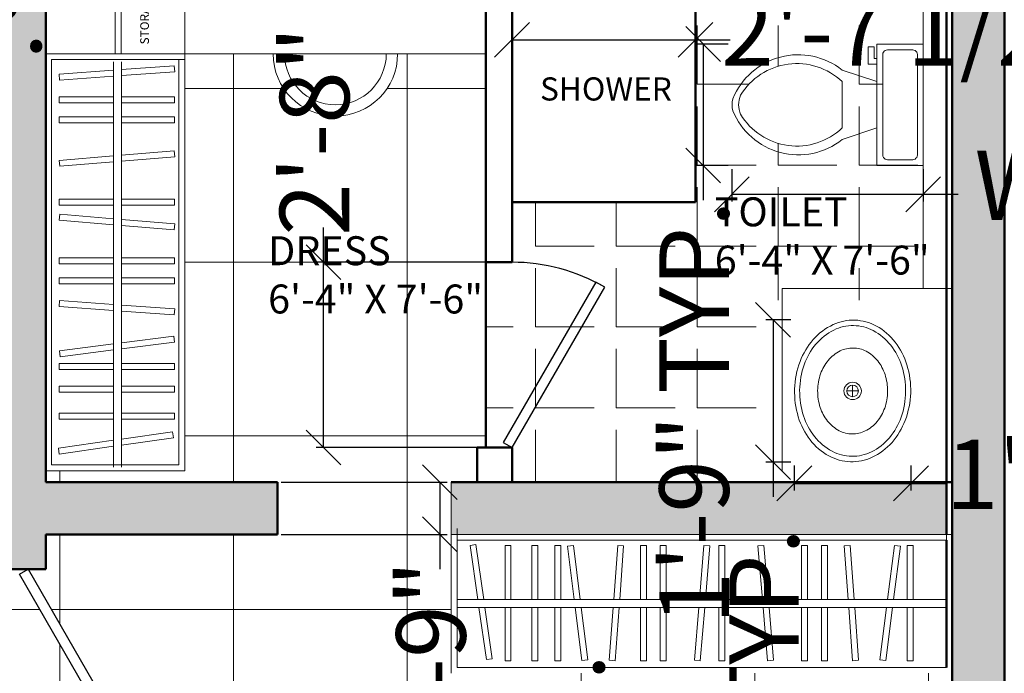
# Model space of a CAD drawing. Units: inches. Extents: x 2371 to 3019, y 129 to 700.
# Tile 12 of 14: x 2753 to 2923, y 499 to 612. Entities that reach past the tile are written whole.
import ezdxf

# ---------------------------------------------------------------- set-up
doc = ezdxf.new("R2010")
doc.units = ezdxf.units.IN
for name, color, linetype, lineweight in [('A-ANNO-DIMS', 2, 'Continuous', 18), ('A-AREA-IDEN', 7, 'Continuous', 25), ('A-DOOR', 4, 'Continuous', 25), ('A-FLOR-FIXT', 8, 'Continuous', 18), ('A-FLOR-PATT', 252, 'Continuous', 13), ('A-FURN', 8, 'Continuous', 18), ('A-WALL', 7, 'Continuous', 50), ('A-WALL-PATT', 8, 'Continuous', 13)]:
    doc.layers.add(name, color=color, linetype=linetype, lineweight=lineweight)
doc.styles.get("Standard").update_dxf_attribs({"font": 'arial.ttf'})
doc.dimstyles.new('ISO-25', dxfattribs={"dimtxt": 12, "dimasz": 6, "dimexe": 1.25, "dimexo": 0.625, "dimtad": 0, "dimdec": 1, "dimlunit": 3, "dimtxsty": 'Standard', "dimblk": 'OBLIQUE', "dimblk1": 'ORIGIN2', "dimblk2": 'OBLIQUE', "dimcen": 2.5, "dimadec": 0, "dimazin": 0, "dimtfac": 1, "dimtdec": 1, "dimtmove": 0, "dimatfit": 3, "dimldrblk": 'OBLIQUE', "dimfxl": 1, "dimarcsym": 0})

# ---------------------------------------------------------------- blocks, each defined once
blk = doc.blocks.new('*U3')
for p, q in [((0, 0), (0, -6)), ((-32, 0), (-32, -6))]:
    blk.add_line(p, q)
blk.add_lwpolyline([(0, 0), (-27.71, 16), (-28.59, 14.48), (-0.88, -1.52)], close=True)
blk.add_arc((0, 0), 32, 150, 180)
blk = doc.blocks.new('*U10')
for p, q in [((0, 0), (0, -6)), ((36, 0), (36, -6))]:
    blk.add_line(p, q)
blk.add_lwpolyline([(0, 0), (31.18, 18), (32.05, 16.48), (0.87, -1.52)], close=True)
blk.add_arc((0, 0), 36, 0, 30)
blk = doc.blocks.new('Sink - Oval top')
for p, q in [((-1, 0), (1, 0)), ((0, 1), (0, -1))]:
    blk.add_line(p, q)
for points in [[(-12.23, 0.39, 0.117634), (-11.46, -3.36, 0.104469), (-8.88, -6.8, 0.090016), (-5.08, -9.07, 0.08192), (-0.32, -10.02, 0.08192), (4.49, -9.38, 0.090016), (8.42, -7.36, 0.104469), (11.22, -4.09, 0.117634), (12.23, -0.39, 0.117634), (11.46, 3.36, 0.104469), (8.88, 6.8, 0.090016), (5.08, 9.07, 0.08192), (0.32, 10.02, 0.08192), (-4.49, 9.38, 0.090016), (-8.42, 7.36, 0.104469), (-11.22, 4.09, 0.117634)], [(-11.29, 0.16, 0.118622), (-10.52, -3.25, 0.104678), (-8.07, -6.36, 0.089562), (-4.54, -8.37, 0.081185), (-0.13, -9.15, 0.081185), (4.3, -8.49, 0.089562), (7.89, -6.58, 0.104678), (10.42, -3.55, 0.118622), (11.29, -0.16, 0.118622), (10.52, 3.25, 0.104678), (8.07, 6.36, 0.089562), (4.54, 8.37, 0.081185), (0.13, 9.15, 0.081185), (-4.3, 8.49, 0.089562), (-7.89, 6.58, 0.104678), (-10.42, 3.55, 0.118622)], [(-7.42, 0.08, 0.118283), (-6.91, -2.17, 0.104607), (-5.29, -4.21, 0.089718), (-2.97, -5.53, 0.081436), (-0.07, -6.04, 0.081436), (2.84, -5.59, 0.089718), (5.2, -4.33, 0.104607), (6.86, -2.32, 0.118283), (7.42, -0.08, 0.118283), (6.91, 2.17, 0.104607), (5.29, 4.21, 0.089718), (2.97, 5.53, 0.081436), (0.07, 6.04, 0.081436), (-2.84, 5.59, 0.089718), (-5.2, 4.33, 0.104607), (-6.86, 2.32, 0.118283)]]:
    blk.add_lwpolyline(points, format="xyb", close=True)
for radius in [1.5, 1]:
    blk.add_circle((0, 0), radius)
blk = doc.blocks.new('Toilet - top')
for p, q in [((9.5, -6), (9.5, -2)), ((-8, -8.5), (-8, -8)), ((-7, -8), (-7, -9.5)), ((-4, -8), (-6, -14)), ((4, -8), (6, -14)), ((-10, -8.5), (-8, -8.5)), ((-10, -9.5), (-10, -8.5)), ((-7, -9.5), (-10, -9.5)), ((4, -14), (-4, -14))]:
    blk.add_line(p, q)
blk.add_lwpolyline([(10.5, -8), (10.5, 0), (-10.5, 0), (-10.5, -8)], close=True)
for points in [[(8.5, -1), (-8.5, -1)], [(-9.5, -2), (-9.5, -6)], [(-8.5, -7), (8.5, -7)]]:
    blk.add_lwpolyline(points)
for centre, radius, start, end in [((-8.62, -1.88), 0.884, 81.8699, 188.1301), ((8.62, -1.88), 0.884, 351.8699, 98.1301), ((-8.62, -6.12), 0.884, 171.8699, 278.1301), ((8.62, -6.12), 0.884, 261.8699, 8.1301), ((3.52, -21.58), 12.17, 141.4691, 247.9714), ((4.2, -21.82), 11.33, 136.3677, 238.9468), ((-3.52, -21.58), 12.17, 292.0284, 38.5307), ((-4.2, -21.82), 11.33, 301.053, 43.6321), ((0, -27.88), 4, 245.7318, 294.2682), ((0, -29), 4, 254.8605, 285.1395)]:
    blk.add_arc(centre, radius, start, end)
blk = doc.blocks.new('_Oblique')
at = {"color": 0, "linetype": 'ByBlock', "lineweight": -2}
blk.add_line((-0.5, -0.5), (0.5, 0.5), dxfattribs=at)
blk = doc.blocks.new('*D25')
at = {"layer": 'A-ANNO-DIMS', "color": 0, "lineweight": -2, "transparency": 16777216}
for p, q in [((2849.61, 422.48), (2849.61, 428.48)), ((2838.23, 422.48), (2850.86, 422.48)), ((2849.61, 362.48), (2849.61, 422.48)), ((2838.23, 362.48), (2850.86, 362.48))]:
    blk.add_line(p, q, dxfattribs=at)
at = {"layer": 'Defpoints', "color": 0, "lineweight": 25, "transparency": 16777216}
for p in [(2837.61, 422.48), (2849.61, 422.48), (2837.61, 362.48)]:
    blk.add_point(p, dxfattribs=at)
at = {"layer": 'A-ANNO-DIMS', "color": 0, "lineweight": -2, "transparency": 16777216, "xscale": 6, "yscale": 6, "zscale": 6}
for p, rotation in [((2849.61, 422.48), 90), ((2849.61, 362.48), 270)]:
    blk.add_blockref('_Oblique', p, dxfattribs=dict(at, rotation=rotation))
at = {"layer": 'A-ANNO-DIMS', "color": 0, "transparency": 16777216, "insert": (2849.61, 465.67), "char_height": 12, "attachment_point": 5, "rotation": 90}
blk.add_mtext('5\'-0" TYP.', dxfattribs=at)
blk = doc.blocks.new('_Origin2')
at = {"color": 0, "linetype": 'ByBlock', "lineweight": -2}
blk.add_line((-0.5, 0), (-1, 0), dxfattribs=at)
for radius in [0.5, 0.25]:
    blk.add_circle((0, 0), radius, dxfattribs=at)
blk = doc.blocks.new('*D26')
at = {"layer": 'A-ANNO-DIMS', "color": 0, "lineweight": -2, "transparency": 16777216}
for p, q in [((2886.23, 560.02), (2881.92, 560.02)), ((2883.17, 560.02), (2883.17, 535.47)), ((2886.23, 535.47), (2881.92, 535.47)), ((2883.17, 535.47), (2883.17, 529.47))]:
    blk.add_line(p, q, dxfattribs=at)
at = {"layer": 'Defpoints', "color": 0, "lineweight": 25, "transparency": 16777216}
for p in [(2886.85, 560.02), (2883.17, 535.47), (2886.85, 535.47)]:
    blk.add_point(p, dxfattribs=at)
at = {"layer": 'A-ANNO-DIMS', "color": 0, "lineweight": -2, "transparency": 16777216, "xscale": 6, "yscale": 6, "zscale": 6}
for p, rotation in [((2883.17, 560.02), 90), ((2883.17, 535.47), 270)]:
    blk.add_blockref('_Oblique', p, dxfattribs=dict(at, rotation=rotation))
at = {"layer": 'A-ANNO-DIMS', "color": 0, "transparency": 16777216, "insert": (2883.17, 423.09), "char_height": 12, "attachment_point": 5, "rotation": 90}
blk.add_mtext('WASH BASIN 2\'-0 1/2" TYP.', dxfattribs=at)
blk = doc.blocks.new('*D27')
at = {"layer": 'A-ANNO-DIMS', "color": 0, "lineweight": -2, "transparency": 16777216}
for p, q in [((2886.85, 534.85), (2886.85, 530.54)), ((2906.99, 534.85), (2906.99, 530.54)), ((2886.85, 531.79), (2906.99, 531.79)), ((2906.99, 531.79), (2912.99, 531.79))]:
    blk.add_line(p, q, dxfattribs=at)
at = {"layer": 'Defpoints', "color": 0, "lineweight": 25, "transparency": 16777216}
for p in [(2886.85, 535.47), (2906.99, 535.47), (2906.99, 531.79)]:
    blk.add_point(p, dxfattribs=at)
at = {"layer": 'A-ANNO-DIMS', "color": 0, "lineweight": -2, "transparency": 16777216, "xscale": 6, "yscale": 6, "zscale": 6, "rotation": 180}
blk.add_blockref('_Oblique', (2886.85, 531.79), dxfattribs=at)
at = {"layer": 'A-ANNO-DIMS', "color": 0, "lineweight": -2, "transparency": 16777216, "xscale": 6, "yscale": 6, "zscale": 6}
blk.add_blockref('_Oblique', (2906.99, 531.79), dxfattribs=at)
at = {"layer": 'A-ANNO-DIMS', "color": 0, "transparency": 16777216, "insert": (2949.62, 531.79), "char_height": 12, "attachment_point": 5}
blk.add_mtext('1\'-8" TYP.', dxfattribs=at)
blk = doc.blocks.new('*D28')
at = {"layer": 'A-ANNO-DIMS', "color": 0, "lineweight": -2, "transparency": 16777216}
for p, q in [((2876.06, 586.05), (2876.06, 580.47)), ((2909.11, 586.05), (2909.11, 580.47)), ((2876.06, 581.72), (2909.11, 581.72)), ((2909.11, 581.72), (2915.11, 581.72))]:
    blk.add_line(p, q, dxfattribs=at)
at = {"layer": 'Defpoints', "color": 0, "lineweight": 25, "transparency": 16777216}
for p in [(2876.06, 586.68), (2909.11, 586.68), (2909.11, 581.72)]:
    blk.add_point(p, dxfattribs=at)
at = {"layer": 'A-ANNO-DIMS', "color": 0, "lineweight": -2, "transparency": 16777216, "xscale": 6, "yscale": 6, "zscale": 6, "rotation": 180}
blk.add_blockref('_Oblique', (2876.06, 581.72), dxfattribs=at)
at = {"layer": 'A-ANNO-DIMS', "color": 0, "lineweight": -2, "transparency": 16777216, "xscale": 6, "yscale": 6, "zscale": 6}
blk.add_blockref('_Oblique', (2909.11, 581.72), dxfattribs=at)
at = {"layer": 'A-ANNO-DIMS', "color": 0, "transparency": 16777216, "insert": (2968.84, 581.72), "char_height": 12, "attachment_point": 5}
blk.add_mtext('WC 2\'-9" TYP.', dxfattribs=at)
blk = doc.blocks.new('*D29')
at = {"layer": 'A-ANNO-DIMS', "color": 0, "lineweight": -2, "transparency": 16777216}
for p, q in [((2875.43, 607.68), (2869.85, 607.68)), ((2871.1, 607.68), (2871.1, 586.68)), ((2875.43, 586.68), (2869.85, 586.68)), ((2871.1, 586.68), (2871.1, 580.68))]:
    blk.add_line(p, q, dxfattribs=at)
at = {"layer": 'Defpoints', "color": 0, "lineweight": 25, "transparency": 16777216}
for p in [(2876.06, 607.68), (2871.1, 586.68), (2876.06, 586.68)]:
    blk.add_point(p, dxfattribs=at)
at = {"layer": 'A-ANNO-DIMS', "color": 0, "lineweight": -2, "transparency": 16777216, "xscale": 6, "yscale": 6, "zscale": 6}
for p, rotation in [((2871.1, 607.68), 90), ((2871.1, 586.68), 270)]:
    blk.add_blockref('_Oblique', p, dxfattribs=dict(at, rotation=rotation))
at = {"layer": 'A-ANNO-DIMS', "color": 0, "transparency": 16777216, "insert": (2871.1, 544.04), "char_height": 12, "attachment_point": 5, "rotation": 90}
blk.add_mtext('1\'-9" TYP.', dxfattribs=at)
blk = doc.blocks.new('*D30')
at = {"layer": 'A-ANNO-DIMS', "color": 0, "lineweight": -2, "transparency": 16777216}
for p, q in [((2505.18, 612.41), (2505.18, 609.58)), ((2519.88, 612.41), (2519.88, 609.58)), ((2505.18, 610.83), (2519.88, 610.83)), ((2519.88, 610.83), (2525.88, 610.83))]:
    blk.add_line(p, q, dxfattribs=at)
at = {"layer": 'Defpoints', "color": 0, "lineweight": 25, "transparency": 16777216}
for p in [(2505.18, 613.03), (2519.88, 613.03), (2519.88, 610.83)]:
    blk.add_point(p, dxfattribs=at)
at = {"layer": 'A-ANNO-DIMS', "color": 0, "lineweight": -2, "transparency": 16777216, "xscale": 6, "yscale": 6, "zscale": 6, "rotation": 180}
blk.add_blockref('_Oblique', (2505.18, 610.83), dxfattribs=at)
at = {"layer": 'A-ANNO-DIMS', "color": 0, "lineweight": -2, "transparency": 16777216, "xscale": 6, "yscale": 6, "zscale": 6}
blk.add_blockref('_Oblique', (2519.88, 610.83), dxfattribs=at)
at = {"layer": 'A-ANNO-DIMS', "color": 0, "transparency": 16777216, "insert": (2645.95, 610.83), "char_height": 12, "attachment_point": 5}
blk.add_mtext('SHOWER MIXER 1\'-2 1/2" TYP.', dxfattribs=at)
blk = doc.blocks.new('*D64')
at = {"layer": 'A-ANNO-DIMS', "color": 0, "lineweight": -2, "transparency": 16777216}
for p, q in [((2798.23, 531.98), (2826.91, 531.98)), ((2825.66, 531.98), (2825.66, 522.98)), ((2798.23, 522.98), (2826.91, 522.98)), ((2825.66, 522.98), (2825.66, 516.98))]:
    blk.add_line(p, q, dxfattribs=at)
at = {"layer": 'Defpoints', "color": 0, "lineweight": 25, "transparency": 16777216}
for p in [(2797.61, 531.98), (2797.61, 522.98), (2825.66, 522.98)]:
    blk.add_point(p, dxfattribs=at)
at = {"layer": 'A-ANNO-DIMS', "color": 0, "lineweight": -2, "transparency": 16777216, "xscale": 6, "yscale": 6, "zscale": 6}
for p, rotation in [((2825.66, 531.98), 90), ((2825.66, 522.98), 270)]:
    blk.add_blockref('_Oblique', p, dxfattribs=dict(at, rotation=rotation))
at = {"layer": 'A-ANNO-DIMS', "color": 0, "transparency": 16777216, "insert": (2825.66, 500.4), "char_height": 12, "attachment_point": 5, "rotation": 90}
blk.add_mtext('0\'-9"', dxfattribs=at)
blk = doc.blocks.new('*D75')
at = {"layer": 'A-ANNO-DIMS', "color": 0, "lineweight": -2, "transparency": 16777216}
for p, q in [((2805.56, 569.98), (2805.56, 575.98)), ((2832.98, 569.98), (2804.31, 569.98)), ((2805.56, 537.98), (2805.56, 569.98)), ((2832.98, 537.98), (2804.31, 537.98))]:
    blk.add_line(p, q, dxfattribs=at)
at = {"layer": 'Defpoints', "color": 0, "lineweight": 25, "transparency": 16777216}
for p in [(2805.56, 569.98), (2833.61, 569.98), (2833.61, 537.98)]:
    blk.add_point(p, dxfattribs=at)
at = {"layer": 'A-ANNO-DIMS', "color": 0, "lineweight": -2, "transparency": 16777216, "xscale": 6, "yscale": 6, "zscale": 6}
for p, rotation in [((2805.56, 569.98), 90), ((2805.56, 537.98), 270)]:
    blk.add_blockref('_Oblique', p, dxfattribs=dict(at, rotation=rotation))
at = {"layer": 'A-ANNO-DIMS', "color": 0, "transparency": 16777216, "insert": (2805.56, 592.65), "char_height": 12, "attachment_point": 5, "rotation": 90}
blk.add_mtext('2\'-8"', dxfattribs=at)
blk = doc.blocks.new('*D77')
at = {"layer": 'A-ANNO-DIMS', "color": 0, "lineweight": -2, "transparency": 16777216}
for p, q in [((2838.11, 580.98), (2838.11, 609.66)), ((2869.78, 580.98), (2869.78, 609.66)), ((2838.11, 608.41), (2869.78, 608.41)), ((2869.78, 608.41), (2875.78, 608.41))]:
    blk.add_line(p, q, dxfattribs=at)
at = {"layer": 'Defpoints', "color": 0, "lineweight": 25, "transparency": 16777216}
for p in [(2869.78, 608.41), (2838.11, 580.36), (2869.78, 580.36)]:
    blk.add_point(p, dxfattribs=at)
at = {"layer": 'A-ANNO-DIMS', "color": 0, "lineweight": -2, "transparency": 16777216, "xscale": 6, "yscale": 6, "zscale": 6, "rotation": 180}
blk.add_blockref('_Oblique', (2838.11, 608.41), dxfattribs=at)
at = {"layer": 'A-ANNO-DIMS', "color": 0, "lineweight": -2, "transparency": 16777216, "xscale": 6, "yscale": 6, "zscale": 6}
blk.add_blockref('_Oblique', (2869.78, 608.41), dxfattribs=at)
at = {"layer": 'A-ANNO-DIMS', "color": 0, "transparency": 16777216, "insert": (2906.44, 608.41), "char_height": 12, "attachment_point": 5}
blk.add_mtext('2\'-7 1/2"', dxfattribs=at)

msp = doc.modelspace()

# ---------------------------------------------------------------- hatches: boundary and pattern name
at = {"layer": 'A-FLOR-PATT'}
h = msp.add_hatch(dxfattribs=at)
h.set_pattern_fill('_USER', color=256, scale=30, pattern_type=0)
h.set_pattern_definition([(0, (0, 0), (0, 30), [])])
h.paths.add_polyline_path([(2913.11, 498.98), (2827.61, 498.98), (2827.61, 531.98), (2832.11, 531.98), (2832.11, 537.98), (2833.61, 537.98), (2833.61, 605.98), (2818.35, 605.98, -1), (2796.86, 605.98), (2781.61, 605.98), (2781.61, 603.98), (2781.61, 533.98), (2757.61, 533.98), (2757.61, 531.98), (2797.61, 531.98), (2797.61, 522.98), (2757.61, 522.98), (2757.61, 516.98), (2754.59, 516.98), (2772.52, 485.76), (2771.01, 484.89), (2770.98, 484.93, -0.097552), (2757.61, 481.1), (2757.61, 422.48), (2837.61, 422.48), (2837.61, 362.48), (2757.61, 362.48), (2757.61, 303.98), (2835.86, 303.98, -0.09439), (2793.86, 311.98), (2793.86, 337.98), (2799.86, 337.98), (2799.86, 336.42), (2871.86, 336.42), (2871.86, 337.98), (2877.86, 337.98), (2877.86, 311.98, -0.09439), (2835.86, 303.98), (2913.11, 303.98), (2913.11, 383.18), (2904.11, 383.18), (2904.11, 419.18), (2913.11, 419.18)])
h.paths.add_polyline_path([(2788.88, 332.88), (2788.88, 308.88), (2764.88, 308.88), (2764.88, 332.88)], flags=16)
h.paths.add_polyline_path([(2788.4, 325.04, -1), (2774.4, 325.04, -1)], flags=0)
h.paths.add_polyline_path([(2781.4, 328.04), (2784.4, 325.04), (2781.4, 322.04), (2778.4, 325.04)], flags=0)
h.paths.add_polyline_path([(2782.4, 325.04, -1), (2780.4, 325.04, -1)], flags=0)
h.paths.add_polyline_path([(2748.61, 480.99), (2754.51, 480.98, 0.119303), (2770.98, 484.93), (2753.07, 516.1), (2754.59, 516.98), (2748.61, 516.98), (2748.61, 539.98), (2712.61, 539.98), (2665.11, 539.98, -0.09439), (2707.11, 531.98), (2707.11, 505.98), (2701.11, 505.98), (2701.11, 507.53), (2629.11, 507.53), (2629.11, 505.98), (2623.11, 505.98), (2623.11, 531.98, -0.09439), (2665.11, 539.98), (2581.61, 539.98), (2581.61, 522.98), (2581.61, 477.98, -0.131044), (2589.61, 507.98), (2615.61, 507.98), (2615.61, 501.98), (2614.05, 501.98), (2614.05, 453.98), (2615.61, 453.98), (2615.61, 447.98), (2589.61, 447.98, -0.131044), (2581.61, 477.98), (2581.61, 432.98), (2572.61, 432.98, 0.119303), (2556.14, 428.99), (2574.12, 397.85), (2572.61, 396.98), (2578.61, 396.98), (2581.61, 396.98), (2581.61, 390.98), (2748.61, 390.98)])
h.paths.add_polyline_path([(2683.1, 447.25), (2652.43, 447.25), (2652.43, 492.22), (2683.1, 492.22)], flags=16)
h.paths.add_polyline_path([(2682.1, 448.25), (2653.43, 448.25), (2653.43, 491.22), (2682.1, 491.22)], flags=0)
h.paths.add_polyline_path([(2613.58, 512.06), (2589.58, 512.06), (2589.58, 536.06), (2613.58, 536.06)], flags=16)
h.paths.add_polyline_path([(2599.1, 528.22, -1), (2613.1, 528.22, -1)], flags=0)
h.paths.add_polyline_path([(2609.1, 528.22), (2606.1, 525.22), (2603.1, 528.22), (2606.1, 531.22)], flags=0)
h.paths.add_polyline_path([(2607.1, 528.22, -1), (2605.1, 528.22, -1)], flags=0)
h.paths.add_polyline_path([(2581.61, 522.98), (2581.61, 621.98), (2572.61, 621.98), (2572.61, 522.98), (2572.61, 500.98), (2565.85, 500.98), (2565.85, 500.15), (2564.82, 500.15), (2561.16, 500.19), (2561.16, 500.17), (2560.13, 500.3), (2560.22, 500.98), (2556.38, 500.98), (2556.43, 500.22), (2555.4, 500.14), (2555.34, 500.98), (2551.07, 500.98), (2551.07, 500.15), (2550.04, 500.15), (2547.64, 500.19), (2547.64, 500.15), (2546.61, 500.15), (2541.79, 500.22), (2540.72, 500.13), (2540.65, 500.98), (2533.37, 500.98), (2533.37, 500.15), (2532.34, 500.15), (2529.13, 500.21), (2529.12, 500.13), (2528.09, 500.22), (2528.16, 500.98), (2523.23, 500.98), (2523.23, 500.15), (2522.2, 500.15), (2519.8, 500.21), (2519.8, 500.15), (2518.77, 500.15), (2514.45, 500.26), (2514.44, 500.14), (2513.41, 500.22), (2513.47, 500.98), (2509.62, 500.98), (2509.71, 500.3), (2508.69, 500.17), (2508.58, 500.98), (2505.03, 500.98), (2505.03, 500.15), (2503.99, 500.15), (2501.07, 500.29), (2501.07, 500.15), (2500.04, 500.15), (2496.44, 500.37), (2496.44, 500.15), (2495.4, 500.15), (2492.55, 500.41), (2492.18, 500.35), (2492.09, 500.98), (2486.11, 500.98), (2486.11, 524.98), (2486.11, 531.98), (2490.61, 531.98), (2490.61, 537.98), (2492.11, 537.98), (2492.11, 605.98), (2476.85, 605.98, -1), (2455.36, 605.98), (2440.11, 605.98), (2440.11, 533.98), (2416.11, 533.98), (2416.11, 605.98), (2416.11, 621.98), (2536.61, 621.98), (2536.61, 630.98), (2407.11, 630.98), (2407.11, 363.98), (2416.11, 363.98), (2416.11, 431.48), (2496.11, 431.48), (2496.11, 371.48), (2416.11, 371.48), (2416.11, 303.98), (2494.36, 303.98, -0.09439), (2452.36, 311.98), (2452.36, 337.98), (2458.36, 337.98), (2458.36, 336.42), (2530.36, 336.42), (2530.36, 337.98), (2536.36, 337.98), (2536.36, 311.98, -0.09439), (2494.36, 303.98), (2572.61, 303.98), (2572.61, 381.98), (2572.61, 396.98), (2554.61, 428.15), (2556.12, 429.03), (2556.14, 428.99, -0.119303), (2572.61, 432.98), (2578.61, 432.98), (2581.61, 432.98)])
h.paths.add_polyline_path([(2450.11, 500.98), (2444.5, 500.98), (2444.44, 500.14), (2443.41, 500.22), (2443.47, 500.98), (2439.62, 500.98), (2439.71, 500.3), (2438.69, 500.17), (2438.58, 500.98), (2435.02, 500.98), (2435.02, 500.15), (2433.99, 500.15), (2433.99, 500.98), (2431.07, 500.98), (2431.07, 500.15), (2430.04, 500.15), (2430.04, 500.98), (2426.43, 500.98), (2426.43, 500.15), (2425.4, 500.15), (2425.4, 500.98), (2423.13, 500.98), (2423.2, 500.5), (2422.18, 500.35), (2422.09, 500.98), (2416.11, 500.98), (2416.11, 524.98), (2416.11, 531.98), (2450.11, 531.98), (2450.11, 522.98)], flags=16)
h.paths.add_polyline_path([(2449.11, 501.98), (2417.11, 501.98), (2417.11, 522.98), (2417.11, 523.98), (2449.11, 523.98)], flags=0)
h.paths.add_polyline_path([(2420.7, 510.73), (2419.36, 520.07), (2420.38, 520.22), (2421.74, 510.73), (2425.4, 510.73), (2425.4, 520.07), (2426.43, 520.07), (2426.43, 510.73), (2430.04, 510.73), (2430.04, 520.07), (2431.07, 520.07), (2431.07, 510.73), (2433.99, 510.73), (2433.99, 520.07), (2435.02, 520.07), (2435.02, 510.73), (2437.35, 510.73), (2436.18, 519.93), (2437.2, 520.06), (2438.39, 510.73), (2444.17, 510.73), (2444.85, 520.08), (2445.88, 520.01), (2445.21, 510.73)], flags=0)
h.paths.add_polyline_path([(2446.94, 336.11), (2446.94, 312.11), (2422.94, 312.11), (2422.94, 336.11)], flags=16)
h.paths.add_polyline_path([(2446.46, 328.27, -1), (2432.46, 328.27, -1)], flags=0)
h.paths.add_polyline_path([(2439.46, 331.27), (2442.46, 328.27), (2439.46, 325.27), (2436.46, 328.27)], flags=0)
h.paths.add_polyline_path([(2440.46, 328.27, -1), (2438.46, 328.27, -1)], flags=0)
h.paths.add_polyline_path([(2816, 444.88), (2866.87, 444.88), (2866.87, 463.54), (2816, 463.54)], flags=24)
h.paths.add_polyline_path([(2794.21, 558.3), (2833.34, 558.3), (2833.34, 576.96), (2794.21, 576.96)], flags=24)
h.paths.add_polyline_path([(2651.69, 411.53), (2711.04, 411.53), (2711.04, 430.19), (2651.69, 430.19)], flags=24)
h.paths.add_polyline_path([(2494.09, 444.88), (2544.97, 444.88), (2544.97, 463.54), (2494.09, 463.54)], flags=24)
h.paths.add_polyline_path([(2444.55, 565.02), (2483.69, 565.02), (2483.69, 583.68), (2444.55, 583.68)], flags=24)
h = msp.add_hatch(dxfattribs=at)
h.set_pattern_fill('_USER', color=256, scale=30, angle=90, pattern_type=0)
h.set_pattern_definition([(90, (0, 0), (-30, 2e-15), [])])
h.paths.add_polyline_path([(2913.11, 498.98), (2827.61, 498.98), (2827.61, 531.98), (2832.11, 531.98), (2832.11, 537.98), (2833.61, 537.98), (2833.61, 605.98), (2818.35, 605.98, -1), (2796.86, 605.98), (2781.61, 605.98), (2781.61, 603.98), (2781.61, 533.98), (2757.61, 533.98), (2757.61, 531.98), (2797.61, 531.98), (2797.61, 522.98), (2757.61, 522.98), (2757.61, 516.98), (2754.59, 516.98), (2772.52, 485.76), (2771.01, 484.89), (2770.98, 484.93, -0.097552), (2757.61, 481.1), (2757.61, 422.48), (2837.61, 422.48), (2837.61, 362.48), (2757.61, 362.48), (2757.61, 303.98), (2835.86, 303.98, -0.09439), (2793.86, 311.98), (2793.86, 337.98), (2799.86, 337.98), (2799.86, 336.42), (2871.86, 336.42), (2871.86, 337.98), (2877.86, 337.98), (2877.86, 311.98, -0.09439), (2835.86, 303.98), (2913.11, 303.98), (2913.11, 383.18), (2904.11, 383.18), (2904.11, 419.18), (2913.11, 419.18)])
h.paths.add_polyline_path([(2788.88, 332.88), (2788.88, 308.88), (2764.88, 308.88), (2764.88, 332.88)], flags=16)
h.paths.add_polyline_path([(2788.4, 325.04, -1), (2774.4, 325.04, -1)], flags=0)
h.paths.add_polyline_path([(2781.4, 328.04), (2784.4, 325.04), (2781.4, 322.04), (2778.4, 325.04)], flags=0)
h.paths.add_polyline_path([(2782.4, 325.04, -1), (2780.4, 325.04, -1)], flags=0)
h.paths.add_polyline_path([(2748.61, 480.99), (2754.51, 480.98, 0.119303), (2770.98, 484.93), (2753.07, 516.1), (2754.59, 516.98), (2748.61, 516.98), (2748.61, 539.98), (2712.61, 539.98), (2665.11, 539.98, -0.09439), (2707.11, 531.98), (2707.11, 505.98), (2701.11, 505.98), (2701.11, 507.53), (2629.11, 507.53), (2629.11, 505.98), (2623.11, 505.98), (2623.11, 531.98, -0.09439), (2665.11, 539.98), (2581.61, 539.98), (2581.61, 522.98), (2581.61, 477.98, -0.131044), (2589.61, 507.98), (2615.61, 507.98), (2615.61, 501.98), (2614.05, 501.98), (2614.05, 453.98), (2615.61, 453.98), (2615.61, 447.98), (2589.61, 447.98, -0.131044), (2581.61, 477.98), (2581.61, 432.98), (2572.61, 432.98, 0.119303), (2556.14, 428.99), (2574.12, 397.85), (2572.61, 396.98), (2578.61, 396.98), (2581.61, 396.98), (2581.61, 390.98), (2748.61, 390.98)])
h.paths.add_polyline_path([(2683.1, 447.25), (2652.43, 447.25), (2652.43, 492.22), (2683.1, 492.22)], flags=16)
h.paths.add_polyline_path([(2682.1, 448.25), (2653.43, 448.25), (2653.43, 491.22), (2682.1, 491.22)], flags=0)
h.paths.add_polyline_path([(2613.58, 512.06), (2589.58, 512.06), (2589.58, 536.06), (2613.58, 536.06)], flags=16)
h.paths.add_polyline_path([(2599.1, 528.22, -1), (2613.1, 528.22, -1)], flags=0)
h.paths.add_polyline_path([(2609.1, 528.22), (2606.1, 525.22), (2603.1, 528.22), (2606.1, 531.22)], flags=0)
h.paths.add_polyline_path([(2607.1, 528.22, -1), (2605.1, 528.22, -1)], flags=0)
h.paths.add_polyline_path([(2581.61, 522.98), (2581.61, 621.98), (2572.61, 621.98), (2572.61, 522.98), (2572.61, 500.98), (2565.85, 500.98), (2565.85, 500.15), (2564.82, 500.15), (2561.16, 500.19), (2561.16, 500.17), (2560.13, 500.3), (2560.22, 500.98), (2556.38, 500.98), (2556.43, 500.22), (2555.4, 500.14), (2555.34, 500.98), (2551.07, 500.98), (2551.07, 500.15), (2550.04, 500.15), (2547.64, 500.19), (2547.64, 500.15), (2546.61, 500.15), (2541.79, 500.22), (2540.72, 500.13), (2540.65, 500.98), (2533.37, 500.98), (2533.37, 500.15), (2532.34, 500.15), (2529.13, 500.21), (2529.12, 500.13), (2528.09, 500.22), (2528.16, 500.98), (2523.23, 500.98), (2523.23, 500.15), (2522.2, 500.15), (2519.8, 500.21), (2519.8, 500.15), (2518.77, 500.15), (2514.45, 500.26), (2514.44, 500.14), (2513.41, 500.22), (2513.47, 500.98), (2509.62, 500.98), (2509.71, 500.3), (2508.69, 500.17), (2508.58, 500.98), (2505.03, 500.98), (2505.03, 500.15), (2503.99, 500.15), (2501.07, 500.29), (2501.07, 500.15), (2500.04, 500.15), (2496.44, 500.37), (2496.44, 500.15), (2495.4, 500.15), (2492.55, 500.41), (2492.18, 500.35), (2492.09, 500.98), (2486.11, 500.98), (2486.11, 524.98), (2486.11, 531.98), (2490.61, 531.98), (2490.61, 537.98), (2492.11, 537.98), (2492.11, 605.98), (2476.85, 605.98, -1), (2455.36, 605.98), (2440.11, 605.98), (2440.11, 533.98), (2416.11, 533.98), (2416.11, 605.98), (2416.11, 621.98), (2536.61, 621.98), (2536.61, 630.98), (2407.11, 630.98), (2407.11, 363.98), (2416.11, 363.98), (2416.11, 431.48), (2496.11, 431.48), (2496.11, 371.48), (2416.11, 371.48), (2416.11, 303.98), (2494.36, 303.98, -0.09439), (2452.36, 311.98), (2452.36, 337.98), (2458.36, 337.98), (2458.36, 336.42), (2530.36, 336.42), (2530.36, 337.98), (2536.36, 337.98), (2536.36, 311.98, -0.09439), (2494.36, 303.98), (2572.61, 303.98), (2572.61, 381.98), (2572.61, 396.98), (2554.61, 428.15), (2556.12, 429.03), (2556.14, 428.99, -0.119303), (2572.61, 432.98), (2578.61, 432.98), (2581.61, 432.98)])
h.paths.add_polyline_path([(2450.11, 500.98), (2444.5, 500.98), (2444.44, 500.14), (2443.41, 500.22), (2443.47, 500.98), (2439.62, 500.98), (2439.71, 500.3), (2438.69, 500.17), (2438.58, 500.98), (2435.02, 500.98), (2435.02, 500.15), (2433.99, 500.15), (2433.99, 500.98), (2431.07, 500.98), (2431.07, 500.15), (2430.04, 500.15), (2430.04, 500.98), (2426.43, 500.98), (2426.43, 500.15), (2425.4, 500.15), (2425.4, 500.98), (2423.13, 500.98), (2423.2, 500.5), (2422.18, 500.35), (2422.09, 500.98), (2416.11, 500.98), (2416.11, 524.98), (2416.11, 531.98), (2450.11, 531.98), (2450.11, 522.98)], flags=16)
h.paths.add_polyline_path([(2449.11, 501.98), (2417.11, 501.98), (2417.11, 522.98), (2417.11, 523.98), (2449.11, 523.98)], flags=0)
h.paths.add_polyline_path([(2420.7, 510.73), (2419.36, 520.07), (2420.38, 520.22), (2421.74, 510.73), (2425.4, 510.73), (2425.4, 520.07), (2426.43, 520.07), (2426.43, 510.73), (2430.04, 510.73), (2430.04, 520.07), (2431.07, 520.07), (2431.07, 510.73), (2433.99, 510.73), (2433.99, 520.07), (2435.02, 520.07), (2435.02, 510.73), (2437.35, 510.73), (2436.18, 519.93), (2437.2, 520.06), (2438.39, 510.73), (2444.17, 510.73), (2444.85, 520.08), (2445.88, 520.01), (2445.21, 510.73)], flags=0)
h.paths.add_polyline_path([(2446.94, 336.11), (2446.94, 312.11), (2422.94, 312.11), (2422.94, 336.11)], flags=16)
h.paths.add_polyline_path([(2446.46, 328.27, -1), (2432.46, 328.27, -1)], flags=0)
h.paths.add_polyline_path([(2439.46, 331.27), (2442.46, 328.27), (2439.46, 325.27), (2436.46, 328.27)], flags=0)
h.paths.add_polyline_path([(2440.46, 328.27, -1), (2438.46, 328.27, -1)], flags=0)
h.paths.add_polyline_path([(2816, 444.88), (2866.87, 444.88), (2866.87, 463.54), (2816, 463.54)], flags=24)
h.paths.add_polyline_path([(2794.21, 558.3), (2833.34, 558.3), (2833.34, 576.96), (2794.21, 576.96)], flags=24)
h.paths.add_polyline_path([(2651.69, 411.53), (2711.04, 411.53), (2711.04, 430.19), (2651.69, 430.19)], flags=24)
h.paths.add_polyline_path([(2494.09, 444.88), (2544.97, 444.88), (2544.97, 463.54), (2494.09, 463.54)], flags=24)
h.paths.add_polyline_path([(2444.55, 565.02), (2483.69, 565.02), (2483.69, 583.68), (2444.55, 583.68)], flags=24)
h = msp.add_hatch(dxfattribs=at)
h.set_pattern_fill('ANGLE', color=256, scale=2)
h.set_pattern_definition([(0, (341.5, 0), (0, 13.97), [10.16, -3.81]), (90, (341.5, 0), (-13.97, 9e-16), [10.16, -3.81])])
h.paths.add_polyline_path([(2909.11, 621.98), (2902.11, 621.98), (2878.11, 621.98), (2869.78, 621.98), (2869.78, 580.36), (2838.11, 580.36), (2838.11, 569.98), (2833.61, 569.98), (2833.61, 537.98), (2838.11, 537.98), (2838.11, 531.98), (2883.14, 531.98), (2883.14, 563.44), (2909.11, 563.44)])
h.paths.add_polyline_path([(2877.58, 595.53, -0.215004), (2877.58, 598.82, -0.48008), (2895.11, 601.18), (2895.11, 593.18, -0.48008)], flags=16)
h.paths.add_polyline_path([(2902.11, 588.68), (2902.11, 605.68, -0.5), (2903.11, 606.68), (2907.11, 606.68, -0.5), (2908.11, 605.68), (2908.11, 588.68, -0.5), (2907.11, 587.68), (2903.11, 587.68, -0.5)], flags=16)
at = {"layer": 'A-WALL-PATT'}
h = msp.add_hatch(color=256, dxfattribs=at)
h.dxf.hatch_style = 1
h.paths.add_polyline_path([(2536.61, 630.98), (2407.11, 630.98), (2407.11, 363.98), (2416.11, 363.98), (2416.11, 498.98), (2416.11, 522.98), (2416.11, 531.98), (2416.11, 603.98), (2416.11, 621.98), (2536.61, 621.98)])
h.paths.add_polyline_path([(2630.98, 630.98), (2560.61, 630.98), (2560.61, 621.98), (2630.98, 621.98)])
h.paths.add_polyline_path([(2878.11, 630.98), (2699.23, 630.98), (2699.23, 621.98), (2878.11, 621.98)])
h.paths.add_polyline_path([(2496.61, 621.98), (2492.11, 621.98), (2492.11, 569.98), (2496.61, 569.98)], flags=17)
h.paths.add_polyline_path([(2581.61, 621.98), (2572.61, 621.98), (2572.61, 522.98), (2572.61, 498.98), (2572.61, 432.98), (2578.61, 432.98), (2581.61, 432.98), (2581.61, 522.98)])
h.paths.add_polyline_path([(2572.61, 531.98), (2486.11, 531.98), (2486.11, 522.98), (2572.61, 522.98)])
h.paths.add_polyline_path([(2450.11, 531.98), (2440.11, 531.98), (2416.11, 531.98), (2416.11, 522.98), (2450.11, 522.98)], flags=17)
h.paths.add_polyline_path([(2416.11, 315.98), (2407.11, 315.98), (2407.11, 294.98), (2458.11, 294.98), (2458.11, 303.98), (2416.11, 303.98)])
h.paths.add_polyline_path([(2757.61, 303.98), (2530.61, 303.98), (2530.61, 294.98), (2757.61, 294.98)])
h.paths.add_polyline_path([(2581.61, 381.98), (2605.61, 381.98), (2617.61, 381.98), (2617.61, 390.98), (2581.61, 390.98), (2581.61, 396.98), (2572.61, 396.98), (2572.61, 381.98), (2572.61, 303.98), (2581.61, 303.98)])
h.paths.add_polyline_path([(2757.61, 480.98), (2748.61, 480.98), (2748.61, 381.98), (2748.61, 303.98), (2757.61, 303.98), (2757.61, 381.98), (2757.61, 422.48)])
h.paths.add_polyline_path([(2797.61, 531.98), (2757.61, 531.98), (2757.61, 603.98), (2757.61, 621.98), (2748.61, 621.98), (2748.61, 516.99), (2754.59, 516.98), (2757.61, 516.98), (2757.61, 522.98), (2797.61, 522.98)])
h.paths.add_polyline_path([(2913.11, 531.98), (2827.61, 531.98), (2827.61, 522.98), (2913.11, 522.98)])
h.paths.add_polyline_path([(2923.11, 630.98), (2902.11, 630.98), (2902.11, 621.98), (2914.11, 621.98), (2914.11, 363.98), (2923.11, 363.98)])
h.paths.add_polyline_path([(2923.11, 315.98), (2914.11, 315.98), (2914.11, 303.98), (2866.11, 303.98), (2866.11, 294.98), (2923.11, 294.98)])
h.paths.add_polyline_path([(2793.61, 303.98), (2757.61, 303.98), (2757.61, 294.98), (2793.61, 294.98)])

# ---------------------------------------------------------------- linework, layer by layer
at = {"layer": 'A-FLOR-FIXT'}
for radius, end in [(10.75, 360), (8.79, 0)]:
    msp.add_arc((2807.61, 605.98), radius, 180, end, dxfattribs=at)
at = {"layer": 'A-FURN'}
for p, q in [((2909.11, 565.44), (2909.11, 623.98)), ((2769.61, 605.98), (2769.61, 621.98)), ((2770.61, 605.98), (2770.61, 620.98)), ((2781.61, 603.98), (2781.61, 621.98)), ((2781.61, 605.98), (2833.61, 605.98)), ((2769.28, 604.59), (2769.28, 534.65)), ((2770.68, 534.65), (2770.68, 604.59)), ((2884.77, 533.98), (2884.77, 565.44)), ((2884.77, 565.44), (2914.11, 565.44)), ((2769.28, 549.09), (2769.28, 534.59)), ((2770.68, 534.59), (2770.68, 549.09)), ((2827.61, 498.98), (2827.61, 531.98)), ((2913.11, 526.62), (2913.11, 499.98)), ((2828.61, 499.98), (2828.61, 523.98)), ((2914.11, 522.98), (2827.61, 522.98)), ((2913.11, 521.98), (2828.61, 521.98)), ((2828.61, 499.98), (2828.61, 521.98)), ((2913.11, 511.73), (2828.66, 511.73)), ((2828.66, 510.33), (2913.11, 510.33)), ((2913.11, 499.98), (2828.61, 499.98))]:
    msp.add_line(p, q, dxfattribs=at)
for points in [[(2781.61, 605.98), (2781.61, 533.98), (2757.61, 533.98), (2757.61, 605.98)], [(2780.61, 604.98), (2780.61, 534.98), (2758.61, 534.98), (2758.61, 604.98)]]:
    msp.add_lwpolyline(points, close=True, dxfattribs=at)
for points in [[(2770.61, 604.98), (2781.61, 604.98)], [(2770.68, 603.26), (2779.79, 603.92), (2779.87, 602.89)], [(2769.28, 602.12), (2760, 601.45), (2759.93, 602.48), (2769.28, 603.16)], [(2779.87, 602.89), (2770.68, 602.22)], [(2769.28, 597.53), (2759.94, 597.53), (2759.94, 598.56), (2769.28, 598.56)], [(2770.68, 598.56), (2779.85, 598.56), (2779.85, 597.53)], [(2779.85, 597.53), (2770.68, 597.53)], [(2769.28, 594.09), (2759.94, 594.09), (2759.94, 595.13), (2769.28, 595.13)], [(2770.68, 595.13), (2779.85, 595.13), (2779.85, 594.09)], [(2779.85, 594.09), (2770.68, 594.09)], [(2769.28, 587.33), (2760.03, 586.56), (2759.94, 587.58), (2769.28, 588.36)], [(2770.68, 588.48), (2779.79, 589.24), (2779.88, 588.21)], [(2779.88, 588.21), (2770.68, 587.44)], [(2769.28, 580.86), (2759.94, 580.86), (2759.94, 579.83), (2769.28, 579.83)], [(2779.85, 580.86), (2770.68, 580.86)], [(2770.68, 579.83), (2779.85, 579.83), (2779.85, 580.86)], [(2769.28, 577.49), (2760.03, 578.26), (2759.94, 577.23), (2769.28, 576.46)], [(2779.88, 576.61), (2770.68, 577.37)], [(2770.68, 576.34), (2779.79, 575.58), (2779.88, 576.61)], [(2769.28, 570.72), (2759.94, 570.72), (2759.94, 569.69), (2769.28, 569.69)], [(2779.85, 570.72), (2770.68, 570.72)], [(2770.68, 569.69), (2779.85, 569.69), (2779.85, 570.72)], [(2769.28, 567.29), (2759.94, 567.29), (2759.94, 566.26), (2769.28, 566.26)], [(2779.85, 567.29), (2770.68, 567.29)], [(2770.68, 566.26), (2779.85, 566.26), (2779.85, 567.29)], [(2769.28, 562.69), (2760, 563.37), (2759.93, 562.34), (2769.28, 561.66)], [(2779.87, 561.93), (2770.68, 562.59)], [(2770.68, 561.56), (2779.79, 560.9), (2779.87, 561.93)], [(2779.71, 557.2), (2770.68, 556.05)], [(2770.68, 555.01), (2779.84, 556.17), (2779.71, 557.2)], [(2769.28, 555.87), (2759.95, 554.69), (2760.08, 553.67), (2769.28, 554.84)], [(2769.28, 552.51), (2759.94, 552.51), (2759.94, 551.48), (2769.28, 551.48)], [(2779.85, 552.51), (2770.68, 552.51)], [(2770.68, 551.48), (2779.85, 551.48), (2779.85, 552.51)], [(2769.28, 548.56), (2759.94, 548.56), (2759.94, 547.53), (2769.28, 547.53)], [(2779.85, 548.56), (2770.68, 548.56)], [(2770.68, 547.53), (2779.85, 547.53), (2779.85, 548.56)], [(2769.28, 543.92), (2759.94, 543.92), (2759.94, 542.89), (2769.28, 542.89)], [(2779.85, 543.92), (2770.68, 543.92)], [(2770.68, 542.89), (2779.85, 542.89), (2779.85, 543.92)], [(2779.51, 540.69), (2770.68, 539.43)], [(2770.68, 538.39), (2779.66, 539.67), (2779.51, 540.69)], [(2769.28, 539.23), (2759.79, 537.87), (2759.94, 536.85), (2769.28, 538.19)], [(2913.11, 527.65), (2913.11, 526.62)], [(2833.24, 511.73), (2831.88, 521.22), (2830.86, 521.07), (2832.2, 511.73)], [(2837.93, 511.73), (2837.93, 521.07), (2836.9, 521.07), (2836.9, 511.73)], [(2842.57, 511.73), (2842.57, 521.07), (2841.54, 521.07), (2841.54, 511.73)], [(2846.52, 511.73), (2846.52, 521.07), (2845.49, 521.07), (2845.49, 511.73)], [(2849.89, 511.73), (2848.7, 521.06), (2847.68, 520.93), (2848.85, 511.73)], [(2856.71, 511.73), (2857.38, 521.01), (2856.35, 521.08), (2855.67, 511.73)], [(2861.3, 511.73), (2861.3, 521.07), (2860.27, 521.07), (2860.27, 511.73)], [(2864.73, 511.73), (2864.73, 521.07), (2863.7, 521.07), (2863.7, 511.73)], [(2871.5, 511.73), (2872.27, 520.98), (2871.24, 521.07), (2870.47, 511.73)], [(2874.87, 511.73), (2874.87, 521.07), (2873.84, 521.07), (2873.84, 511.73)], [(2881.34, 511.73), (2880.57, 520.98), (2881.6, 521.07), (2882.37, 511.73)], [(2888.11, 511.73), (2888.11, 521.07), (2889.14, 521.07), (2889.14, 511.73)], [(2891.54, 511.73), (2891.54, 521.07), (2892.57, 521.07), (2892.57, 511.73)], [(2896.14, 511.73), (2895.46, 521.01), (2896.49, 521.08), (2897.17, 511.73)], [(2902.95, 511.73), (2904.14, 521.06), (2905.16, 520.93), (2903.99, 511.73)], [(2906.32, 511.73), (2906.32, 521.07), (2907.35, 521.07), (2907.35, 511.73)], [(2832.4, 510.33), (2833.68, 501.35), (2834.7, 501.5)], [(2834.7, 501.5), (2833.44, 510.33)], [(2836.9, 510.33), (2836.9, 501.15), (2837.93, 501.15)], [(2837.93, 501.15), (2837.93, 510.33)], [(2841.54, 510.33), (2841.54, 501.15), (2842.57, 501.15)], [(2842.57, 501.15), (2842.57, 510.33)], [(2845.49, 510.33), (2845.49, 501.15), (2846.52, 501.15)], [(2846.52, 501.15), (2846.52, 510.33)], [(2849.02, 510.33), (2850.19, 501.17), (2851.21, 501.3)], [(2851.21, 501.3), (2850.06, 510.33)], [(2855.57, 510.33), (2854.91, 501.22), (2855.94, 501.14)], [(2855.94, 501.14), (2856.6, 510.33)], [(2860.27, 510.33), (2860.27, 501.15), (2861.3, 501.15)], [(2861.3, 501.15), (2861.3, 510.33)], [(2863.7, 510.33), (2863.7, 501.15), (2864.73, 501.15)], [(2864.73, 501.15), (2864.73, 510.33)], [(2870.35, 510.33), (2869.59, 501.22), (2870.62, 501.13)], [(2870.62, 501.13), (2871.38, 510.33)], [(2873.84, 510.33), (2873.84, 501.15), (2874.87, 501.15)], [(2874.87, 501.15), (2874.87, 510.33)], [(2882.22, 501.13), (2881.46, 510.33)], [(2882.49, 510.33), (2883.25, 501.22), (2882.22, 501.13)], [(2888.11, 501.15), (2888.11, 510.33)], [(2889.14, 510.33), (2889.14, 501.15), (2888.11, 501.15)], [(2892.57, 510.33), (2892.57, 501.15), (2891.54, 501.15)], [(2891.54, 501.15), (2891.54, 510.33)], [(2896.9, 501.14), (2896.24, 510.33)], [(2897.27, 510.33), (2897.93, 501.22), (2896.9, 501.14)], [(2903.82, 510.33), (2902.66, 501.17), (2901.63, 501.3)], [(2901.63, 501.3), (2902.78, 510.33)], [(2907.35, 510.33), (2907.35, 501.15), (2906.32, 501.15)], [(2906.32, 501.15), (2906.32, 510.33)]]:
    msp.add_lwpolyline(points, dxfattribs=at)
at = {"layer": 'A-WALL'}
for p, q in [((2923.11, 294.98), (2923.11, 630.98)), ((2757.61, 531.98), (2757.61, 621.98)), ((2833.61, 537.98), (2833.61, 621.98)), ((2838.11, 569.98), (2838.11, 621.98)), ((2869.78, 621.98), (2869.78, 580.36)), ((2913.11, 522.98), (2913.11, 621.98)), ((2914.11, 303.98), (2914.11, 621.98)), ((2869.78, 580.36), (2838.11, 580.36)), ((2838.11, 569.98), (2833.61, 569.98)), ((2838.11, 537.98), (2832.11, 537.98)), ((2832.11, 537.98), (2832.11, 531.98)), ((2838.11, 531.98), (2838.11, 537.98)), ((2797.61, 531.98), (2757.61, 531.98)), ((2797.61, 522.98), (2797.61, 531.98)), ((2914.11, 531.98), (2827.61, 531.98)), ((2797.61, 522.98), (2757.61, 522.98)), ((2757.61, 516.98), (2757.61, 522.98)), ((2913.11, 499.98), (2913.11, 521.98)), ((2757.61, 516.98), (2748.61, 516.98))]:
    msp.add_line(p, q, dxfattribs=at)

# ---------------------------------------------------------------- block references
at = {"layer": 'A-DOOR'}
for name, p, rotation in [('*U3', (2838.11, 537.98), 270), ('*U10', (2754.59, 516.98), 269.8782938999684)]:
    msp.add_blockref(name, p, dxfattribs=dict(at, rotation=rotation))
at = {"layer": 'A-FLOR-FIXT', "rotation": 270}
for name, p in [('Toilet - top', (2909.11, 597.18)), ('Sink - Oval top', (2896.92, 547.75))]:
    msp.add_blockref(name, p, dxfattribs=at)

# ---------------------------------------------------------------- texts
at = {"layer": 'A-AREA-IDEN', "insert": (2773.92, 607.61), "char_height": 1.5, "attachment_point": 1, "rotation": 90}
msp.add_mtext_dynamic_manual_height_columns('STORAGE', width=1.7945, gutter_width=12.5, heights=[0], dxfattribs=at)
at = {"layer": 'A-AREA-IDEN', "ltscale": 2, "attachment_point": 1}
for s, insert, char_height in [('SHOWER', (2842.95, 601.92), 4), ('TOILET\\P6\'-4" X 7\'-6"', (2873.11, 581.19), 5), ('DRESS\\P6\'-4" X 7\'-6"', (2796, 574.47), 5)]:
    msp.add_mtext_dynamic_manual_height_columns(s, width=39.2097, gutter_width=12.5, heights=[0], dxfattribs=dict(at, insert=insert, char_height=char_height))

# ---------------------------------------------------------------- dimensions: what is measured, and where the dimension line sits
at = {"layer": 'A-ANNO-DIMS'}
for base, p1, p2, text, picture, middle in [((2519.88, 610.83), (2505.18, 613.03), (2519.88, 613.03), 'SHOWER MIXER <> TYP.', '*D30', (2645.95, 610.83)), ((2909.1051, 581.7183), (2876.0589, 586.6753), (2909.1051, 586.6753), 'WC <> TYP.', '*D28', (2968.842, 581.7183)), ((2906.99, 531.79), (2886.85, 535.47), (2906.99, 535.47), '<> TYP.', '*D27', (2949.62, 531.79))]:
    dim = msp.add_linear_dim(base=base, p1=p1, p2=p2, text=text, dimstyle='ISO-25', override={"dimdec": 1, "dimrnd": 0, "dimzin": 1, "dimlunit": 4, "dimfrac": 2}, dxfattribs=at)
    dim.commit()
    dim.dimension.update_dxf_attribs({"geometry": picture, "text_midpoint": middle})
for base, p1, p2, angle, picture, middle in [((2869.78, 608.41), (2838.11, 580.36), (2869.78, 580.36), 0, '*D77', (2906.44, 608.41)), ((2805.56, 569.98), (2833.61, 537.98), (2833.61, 569.98), 90, '*D75', (2805.56, 592.65)), ((2825.66, 522.98), (2797.61, 531.98), (2797.61, 522.98), 270, '*D64', (2825.66, 500.4))]:
    dim = msp.add_linear_dim(base=base, p1=p1, p2=p2, angle=angle, dimstyle='ISO-25', override={"dimdec": 1, "dimlfac": 1, "dimrnd": 0, "dimzin": 1, "dimdsep": 46, "dimlunit": 4, "dimfrac": 2}, dxfattribs=at)
    dim.commit()
    dim.dimension.update_dxf_attribs({"geometry": picture, "text_midpoint": middle})
for base, p1, p2, angle, text, picture, middle in [((2871.1, 586.68), (2876.06, 607.68), (2876.06, 586.68), 270, '<> TYP.', '*D29', (2871.1, 544.04)), ((2883.1676, 535.4732), (2886.8502, 560.0241), (2886.8502, 535.4732), 270, 'WASH BASIN <> TYP.', '*D26', (2883.1676, 423.0911)), ((2849.61, 422.48), (2837.61, 362.48), (2837.61, 422.48), 90, '<> TYP.', '*D25', (2849.61, 465.67))]:
    dim = msp.add_linear_dim(base=base, p1=p1, p2=p2, angle=angle, text=text, dimstyle='ISO-25', override={"dimdec": 1, "dimrnd": 0, "dimzin": 1, "dimlunit": 4, "dimfrac": 2}, dxfattribs=at)
    dim.commit()
    dim.dimension.update_dxf_attribs({"geometry": picture, "text_midpoint": middle})

doc.saveas('drawing.dxf')
